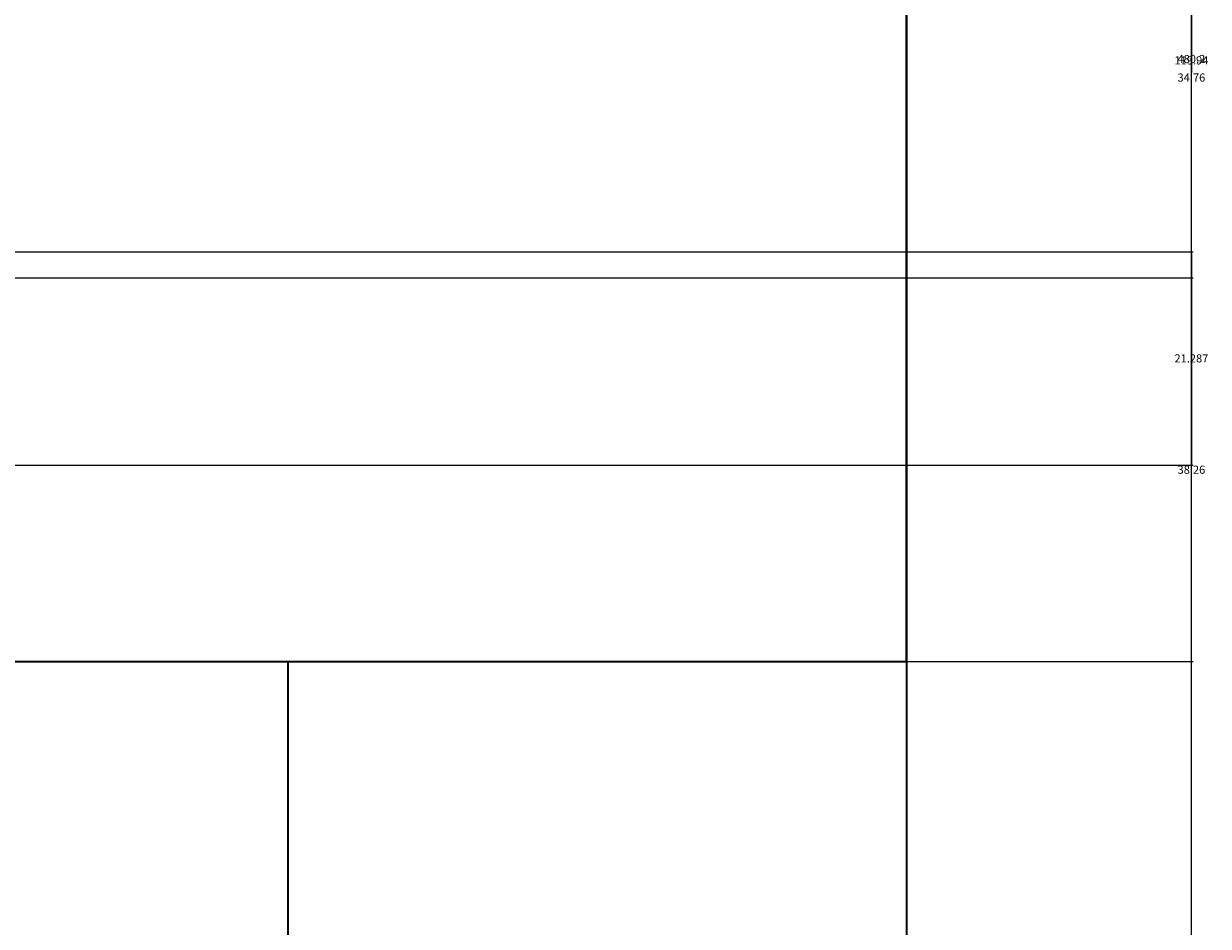
# Model space of a CAD drawing. Units: inches. Extents: x 69 to 650, y -16 to 573.
# Tile 21 of 26: x 531 to 650, y 218 to 308. Entities that reach past the tile are written whole.
import ezdxf

# ---------------------------------------------------------------- set-up
doc = ezdxf.new("R2010")
doc.units = ezdxf.units.IN
doc.header["$MEASUREMENT"] = 0
doc.layers.add('A-ANNO-DIMS', color=2, linetype='Continuous', lineweight=18)
doc.layers.add('A-WALL', color=7, linetype='Continuous', lineweight=35)
doc.styles.get("Standard").update_dxf_attribs({"font": 'arial.ttf'})
doc.dimstyles.get("Standard").update_dxf_attribs({"dimtxt": 0.8125, "dimasz": 0.18, "dimexe": 0.18, "dimexo": 0.0625, "dimgap": 0.09, "dimtad": 0, "dimtih": 1, "dimtoh": 1, "dimdec": 4, "dimzin": 0, "dimdsep": 46, "dimlunit": 4, "dimtxsty": 'Standard', "dimcen": 0.09, "dimadec": 0, "dimazin": 0, "dimtfac": 1, "dimtdec": 4, "dimtofl": 0, "dimtmove": 0, "dimatfit": 3, "dimfxl": 1, "dimtolj": 1, "dimtzin": 0, "dimarcsym": 0})

# ---------------------------------------------------------------- blocks, each defined once
blk = doc.blocks.new('*D19')
at = {"layer": 'A-ANNO-DIMS', "color": 0, "lineweight": -2, "transparency": 16777216}
for p, q in [((99.56, 471.72), (99.56, 572.74)), ((99.74, 572.56), (358.57, 572.56)), ((619.38, 572.56), (360.54, 572.56)), ((619.56, 87.99), (619.56, 572.74))]:
    blk.add_line(p, q, dxfattribs=at)
at = {"layer": 'A-ANNO-DIMS', "color": 0, "transparency": 16777216}
for points in [[(99.74, 572.59), (99.74, 572.53), (99.56, 572.56)], [(619.38, 572.59), (619.38, 572.53), (619.56, 572.56)]]:
    blk.add_solid(points, dxfattribs=at)
at = {"layer": 'Defpoints', "color": 0, "transparency": 16777216}
for p in [(619.56, 572.56), (99.56, 471.66), (619.56, 87.93)]:
    blk.add_point(p, dxfattribs=at)
at = {"layer": 'A-ANNO-DIMS', "color": 0, "transparency": 16777216, "insert": (359.56, 572.56), "char_height": 0.812, "attachment_point": 5}
blk.add_mtext('\\A1;520', dxfattribs=at)
blk = doc.blocks.new('*D20')
at = {"layer": 'A-ANNO-DIMS', "color": 0, "lineweight": -2, "transparency": 16777216}
for p, q in [((504.24, 544.16), (648.14, 544.16)), ((647.96, 543.98), (647.96, 304.55)), ((647.96, 64.11), (647.96, 303.54)), ((619.62, 63.93), (648.14, 63.93))]:
    blk.add_line(p, q, dxfattribs=at)
at = {"layer": 'A-ANNO-DIMS', "color": 0, "transparency": 16777216}
for points in [[(647.93, 543.98), (647.99, 543.98), (647.96, 544.16)], [(647.93, 64.11), (647.99, 64.11), (647.96, 63.93)]]:
    blk.add_solid(points, dxfattribs=at)
at = {"layer": 'Defpoints', "color": 0, "transparency": 16777216}
for p in [(504.18, 544.16), (647.96, 544.16), (619.56, 63.93)]:
    blk.add_point(p, dxfattribs=at)
at = {"layer": 'A-ANNO-DIMS', "color": 0, "transparency": 16777216, "insert": (647.96, 304.04), "char_height": 0.812, "attachment_point": 5}
blk.add_mtext('\\A1;480.2', dxfattribs=at)
blk = doc.blocks.new('*D41')
at = {"layer": 'A-ANNO-DIMS', "color": 0, "lineweight": -2, "transparency": 16777216}
for p, q in [((528.81, 243.87), (528.81, 35.35)), ((619.56, 243.87), (619.56, 35.35)), ((528.99, 35.53), (572.72, 35.53)), ((619.38, 35.53), (575.64, 35.53))]:
    blk.add_line(p, q, dxfattribs=at)
at = {"layer": 'A-ANNO-DIMS', "color": 0, "transparency": 16777216}
for points in [[(528.99, 35.56), (528.99, 35.5), (528.81, 35.53)], [(619.38, 35.56), (619.38, 35.5), (619.56, 35.53)]]:
    blk.add_solid(points, dxfattribs=at)
at = {"layer": 'Defpoints', "color": 0, "transparency": 16777216}
for p in [(528.81, 243.93), (619.56, 243.93), (619.56, 35.53)]:
    blk.add_point(p, dxfattribs=at)
at = {"layer": 'A-ANNO-DIMS', "color": 0, "transparency": 16777216, "insert": (574.18, 35.53), "char_height": 0.812, "attachment_point": 5}
blk.add_mtext('\\A1;90.74', dxfattribs=at)
blk = doc.blocks.new('*D42')
at = {"layer": 'A-ANNO-DIMS', "color": 0, "lineweight": -2, "transparency": 16777216}
for p, q in [((502.63, 282.19), (648.14, 282.19)), ((647.96, 282.01), (647.96, 263.57)), ((647.96, 244.11), (647.96, 262.56)), ((507.67, 243.93), (648.14, 243.93))]:
    blk.add_line(p, q, dxfattribs=at)
at = {"layer": 'A-ANNO-DIMS', "color": 0, "transparency": 16777216}
for points in [[(647.93, 282.01), (647.99, 282.01), (647.96, 282.19)], [(647.93, 244.11), (647.99, 244.11), (647.96, 243.93)]]:
    blk.add_solid(points, dxfattribs=at)
at = {"layer": 'Defpoints', "color": 0, "transparency": 16777216}
for p in [(502.56, 282.19), (647.96, 282.19), (507.61, 243.93)]:
    blk.add_point(p, dxfattribs=at)
at = {"layer": 'A-ANNO-DIMS', "color": 0, "transparency": 16777216, "insert": (647.96, 263.06), "char_height": 0.812, "attachment_point": 5}
blk.add_mtext('\\A1;38.26', dxfattribs=at)
blk = doc.blocks.new('*D43')
at = {"layer": 'A-ANNO-DIMS', "color": 0, "lineweight": -2, "transparency": 16777216}
for p, q in [((502.63, 353.14), (648.14, 353.14)), ((647.96, 352.96), (647.96, 318.17)), ((647.96, 282.37), (647.96, 317.16)), ((502.63, 282.19), (648.14, 282.19))]:
    blk.add_line(p, q, dxfattribs=at)
at = {"layer": 'A-ANNO-DIMS', "color": 0, "transparency": 16777216}
for points in [[(647.93, 352.96), (647.99, 352.96), (647.96, 353.14)], [(647.93, 282.37), (647.99, 282.37), (647.96, 282.19)]]:
    blk.add_solid(points, dxfattribs=at)
at = {"layer": 'Defpoints', "color": 0, "transparency": 16777216}
for p in [(502.56, 353.14), (647.96, 353.14), (502.56, 282.19)]:
    blk.add_point(p, dxfattribs=at)
at = {"layer": 'A-ANNO-DIMS', "color": 0, "transparency": 16777216, "insert": (647.96, 317.67), "char_height": 0.812, "attachment_point": 5}
blk.add_mtext('\\A1;70.95', dxfattribs=at)
blk = doc.blocks.new('*D46')
at = {"layer": 'A-ANNO-DIMS', "color": 0, "lineweight": -2, "transparency": 16777216}
for p, q in [((619.62, 363.87), (648.14, 363.87)), ((647.96, 363.69), (647.96, 304.41)), ((647.96, 244.11), (647.96, 303.4)), ((619.62, 243.93), (648.14, 243.93))]:
    blk.add_line(p, q, dxfattribs=at)
at = {"layer": 'A-ANNO-DIMS', "color": 0, "transparency": 16777216}
for points in [[(647.93, 363.69), (647.99, 363.69), (647.96, 363.87)], [(647.93, 244.11), (647.99, 244.11), (647.96, 243.93)]]:
    blk.add_solid(points, dxfattribs=at)
at = {"layer": 'Defpoints', "color": 0, "transparency": 16777216}
for p in [(619.56, 363.87), (647.96, 363.87), (619.56, 243.93)]:
    blk.add_point(p, dxfattribs=at)
at = {"layer": 'A-ANNO-DIMS', "color": 0, "transparency": 16777216, "insert": (647.96, 303.9), "char_height": 0.812, "attachment_point": 5}
blk.add_mtext('\\A1;119.94', dxfattribs=at)
blk = doc.blocks.new('*D72')
at = {"layer": 'A-ANNO-DIMS', "color": 0, "lineweight": -2, "transparency": 16777216}
for p, q in [((383.36, 284.81), (648.14, 284.81)), ((647.96, 284.63), (647.96, 274.67)), ((647.96, 263.71), (647.96, 273.66)), ((383.36, 263.53), (648.14, 263.53))]:
    blk.add_line(p, q, dxfattribs=at)
at = {"layer": 'A-ANNO-DIMS', "color": 0, "transparency": 16777216}
for points in [[(647.93, 284.63), (647.99, 284.63), (647.96, 284.81)], [(647.93, 263.71), (647.99, 263.71), (647.96, 263.53)]]:
    blk.add_solid(points, dxfattribs=at)
at = {"layer": 'Defpoints', "color": 0, "transparency": 16777216}
for p in [(383.3, 284.81), (647.96, 284.81), (383.3, 263.53)]:
    blk.add_point(p, dxfattribs=at)
at = {"layer": 'A-ANNO-DIMS', "color": 0, "transparency": 16777216, "insert": (647.96, 274.17), "char_height": 0.812, "attachment_point": 5}
blk.add_mtext('\\A1;21.287', dxfattribs=at)
blk = doc.blocks.new('*D73')
at = {"layer": 'A-ANNO-DIMS', "color": 0, "lineweight": -2, "transparency": 16777216}
for p, q in [((383.36, 319.57), (648.14, 319.57)), ((647.96, 319.39), (647.96, 302.7)), ((647.96, 284.99), (647.96, 301.69)), ((383.36, 284.81), (648.14, 284.81))]:
    blk.add_line(p, q, dxfattribs=at)
at = {"layer": 'A-ANNO-DIMS', "color": 0, "transparency": 16777216}
for points in [[(647.93, 319.39), (647.99, 319.39), (647.96, 319.57)], [(647.93, 284.99), (647.99, 284.99), (647.96, 284.81)]]:
    blk.add_solid(points, dxfattribs=at)
at = {"layer": 'Defpoints', "color": 0, "transparency": 16777216}
for p in [(383.3, 319.57), (647.96, 319.57), (383.3, 284.81)]:
    blk.add_point(p, dxfattribs=at)
at = {"layer": 'A-ANNO-DIMS', "color": 0, "transparency": 16777216, "insert": (647.96, 302.19), "char_height": 0.812, "attachment_point": 5}
blk.add_mtext('\\A1;34.76', dxfattribs=at)

msp = doc.modelspace()

# ---------------------------------------------------------------- linework, layer by layer
at = {"layer": 'A-WALL'}
for p, q in [((619.555, 411.93), (619.555, 69.3788)), ((99.556, 243.93), (619.555, 243.93)), ((557.8179, 243.93), (557.8179, 87.93))]:
    msp.add_line(p, q, dxfattribs=at)
msp.add_lwpolyline([(619.555, 363.8739), (528.812, 363.8739), (528.812, 243.93), (619.555, 243.93)], close=True, dxfattribs=at)

# ---------------------------------------------------------------- dimensions: what is measured, and where the dimension line sits
at = {"layer": 'A-ANNO-DIMS'}
for base, p1, p2, override, picture, middle in [((619.555, 572.5573), (99.556, 471.6595), (619.555, 87.93), {"dimdec": 0, "dimlfac": 1, "dimrnd": 0, "dimzin": 0, "dimdsep": 46, "dimlunit": 2}, '*D19', (359.5555, 572.5573)), ((619.555, 35.53), (528.812, 243.93), (619.555, 243.93), {"dimdec": 2, "dimlfac": 1, "dimrnd": 0, "dimzin": 0, "dimdsep": 46, "dimlunit": 2}, '*D41', (574.1835, 35.53))]:
    dim = msp.add_linear_dim(base=base, p1=p1, p2=p2, dimstyle='Standard', override=override, dxfattribs=at)
    dim.commit()
    dim.dimension.update_dxf_attribs({"geometry": picture, "text_midpoint": middle})
for base, p1, p2, override, picture, middle in [((647.955, 544.1573), (619.555, 63.93), (504.1763, 544.1573), {"dimdec": 1, "dimlfac": 1, "dimrnd": 0, "dimzin": 0, "dimdsep": 46, "dimlunit": 2}, '*D20', (647.955, 304.0436)), ((647.955, 363.8739), (619.555, 243.93), (619.555, 363.8739), {"dimdec": 2, "dimlfac": 1, "dimrnd": 0, "dimzin": 0, "dimdsep": 46, "dimlunit": 2}, '*D46', (647.955, 303.902)), ((647.955, 353.1381), (502.5637, 282.1923), (502.5637, 353.1381), {"dimdec": 2, "dimlfac": 1, "dimrnd": 0, "dimzin": 0, "dimdsep": 46, "dimlunit": 2}, '*D43', (647.955, 317.6652)), ((647.955, 319.5737), (383.3022, 284.812), (383.3022, 319.5737), {"dimdec": 2, "dimlfac": 1, "dimrnd": 0, "dimzin": 0, "dimdsep": 46, "dimlunit": 2}, '*D73', (647.955, 302.1928)), ((647.955, 284.812), (383.3022, 263.5253), (383.3022, 284.812), {"dimdec": 3, "dimlfac": 1, "dimrnd": 0, "dimzin": 0, "dimdsep": 46, "dimlunit": 2}, '*D72', (647.955, 274.1686)), ((647.955, 282.1923), (507.611, 243.93), (502.5637, 282.1923), {"dimdec": 2, "dimlfac": 1, "dimrnd": 0, "dimzin": 0, "dimdsep": 46, "dimlunit": 2}, '*D42', (647.955, 263.0612))]:
    dim = msp.add_linear_dim(base=base, p1=p1, p2=p2, angle=90, dimstyle='Standard', override=override, dxfattribs=at)
    dim.commit()
    dim.dimension.update_dxf_attribs({"geometry": picture, "text_midpoint": middle})

doc.saveas('drawing.dxf')
